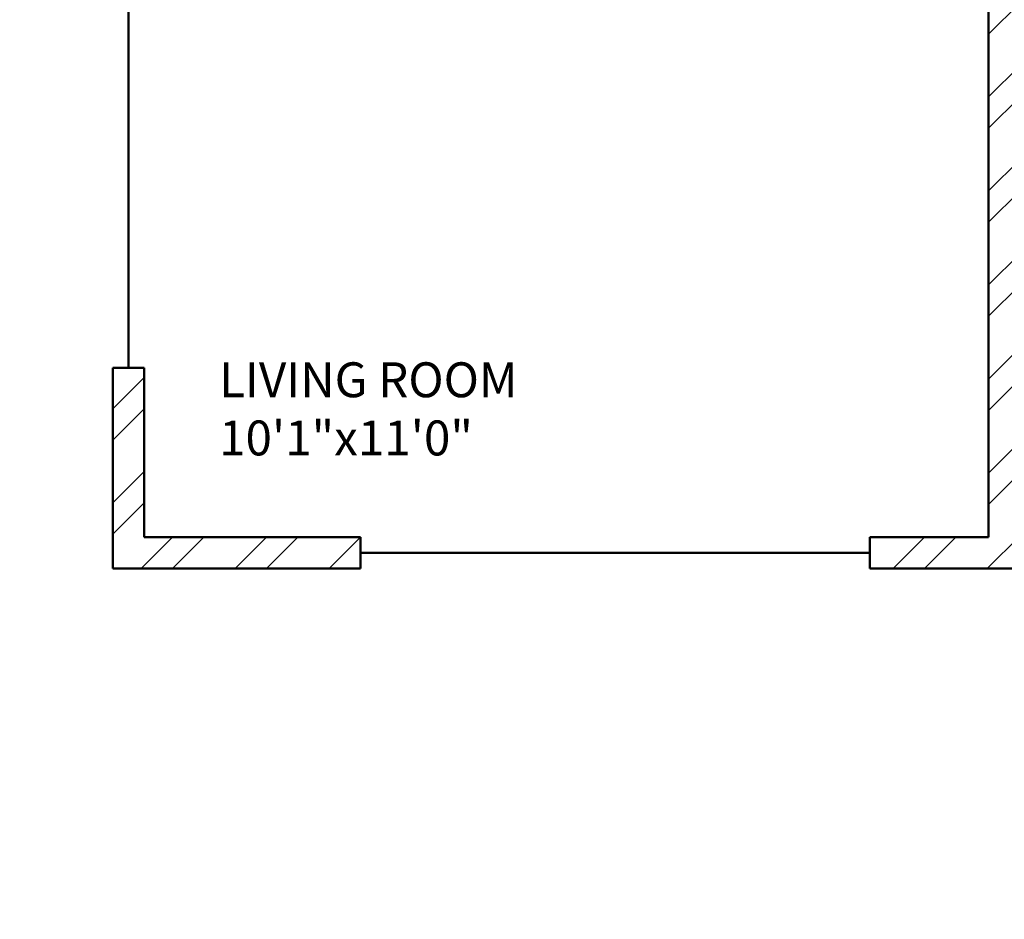
# Model space of a CAD drawing. Units: inches. Extents: x 1901 to 2863, y 888 to 2433.
# Tile 36 of 91: x 2477 to 2618, y 1474 to 1603. Entities that reach past the tile are written whole.
import ezdxf

# ---------------------------------------------------------------- set-up
doc = ezdxf.new("R2010")
doc.units = ezdxf.units.IN
for name, color, linetype, lineweight in [('A-AREA-IDEN', 7, 'Continuous', 18), ('A-WALL', 7, 'Continuous', 50), ('A-WALL-PATT', 8, 'Continuous', 13)]:
    doc.layers.add(name, color=color, linetype=linetype, lineweight=lineweight)
doc.styles.get("Standard").update_dxf_attribs({"font": 'arial.ttf'})

msp = doc.modelspace()

# ---------------------------------------------------------------- hatches: boundary and pattern name
at = {"layer": 'A-WALL-PATT'}
h = msp.add_hatch(dxfattribs=at)
h.set_pattern_fill('ANSI32', color=256)
h.paths.add_polyline_path([(2192.5, 2274.13), (2141.26, 2274.13), (2141.26, 2269.63), (2192.5, 2269.63)])
h.paths.add_polyline_path([(2259.93, 2274.13), (2216.5, 2274.13), (2216.5, 2269.63), (2255.43, 2269.63), (2255.43, 2214.63), (2250.81, 2214.63), (2250.81, 2210.13), (2259.93, 2210.13), (2259.93, 2215.13), (2271.76, 2215.13), (2271.76, 2217.38), (2271.76, 2219.63), (2259.93, 2219.63)])
h.paths.add_polyline_path([(2171.43, 2269.63), (2166.93, 2269.63), (2166.93, 2219.63), (2121.24, 2219.63), (2121.24, 2215.13), (2166.93, 2215.13), (2166.93, 2083.13), (2161.81, 2083.13), (2161.81, 2078.63), (2171.43, 2078.63), (2177, 2078.63), (2177, 2080.88), (2177, 2083.13), (2171.43, 2083.13), (2171.43, 2210.13), (2230.91, 2210.13), (2230.91, 2212.38), (2230.91, 2214.63), (2171.43, 2214.63)])
h.paths.add_polyline_path([(2117.26, 2274.13), (2089.43, 2274.13), (2089.43, 2219.63), (2081.14, 2219.63), (2081.14, 2215.13), (2089.43, 2215.13), (2098, 2215.13), (2098, 2217.38), (2098, 2219.63), (2093.93, 2219.63), (2093.93, 2269.63), (2117.26, 2269.63), (2117.26, 2271.88)])
h.paths.add_polyline_path([(2343.43, 2219.63), (2329.29, 2219.63), (2329.29, 2215.13), (2338.93, 2215.13), (2338.93, 2184.74), (2343.43, 2184.74)])
h.paths.add_polyline_path([(2338.93, 2083.13), (2329.29, 2083.13), (2208.97, 2083.13), (2208.97, 2078.63), (2338.93, 2078.63)])
h.paths.add_polyline_path([(2343.43, 2136.74), (2338.93, 2136.74), (2338.93, 1872.63), (2343.43, 1872.63)])
h.paths.add_polyline_path([(2343.43, 1863.63), (2397.68, 1863.63), (2397.68, 1821.63), (2384.14, 1821.63), (2384.14, 1812.63), (2418.33, 1812.63), (2418.33, 1817.13), (2418.33, 1821.63), (2406.68, 1821.63), (2406.68, 1863.63), (2459.5, 1863.63), (2459.5, 1821.63), (2447.14, 1821.63), (2447.14, 1812.63), (2459.5, 1812.63), (2468.5, 1812.63), (2468.5, 1872.63), (2394.43, 1872.63), (2334.43, 1872.63), (2334.43, 1812.63), (2343.43, 1812.63), (2353.25, 1812.63), (2353.25, 1821.63), (2343.43, 1821.63)])
h.paths.add_polyline_path([(2510.01, 1872.63), (2468.5, 1872.63), (2468.5, 1868.13), (2510.01, 1868.13)])
h.paths.add_polyline_path([(2514.01, 1817.13), (2468.5, 1817.13), (2468.5, 1812.63), (2482.11, 1812.63), (2482.11, 1800.61), (2486.61, 1800.61), (2486.61, 1812.63), (2514.01, 1812.63)])
h.paths.add_polyline_path([(2299.25, 1814.88), (2299.25, 1817.13), (2295.93, 1817.13), (2295.93, 1854.17), (2293.68, 1854.17), (2291.43, 1854.17), (2291.43, 1817.13), (2266.11, 1817.13), (2266.11, 1812.63), (2299.25, 1812.63)])
h.paths.add_polyline_path([(2218.11, 1817.13), (2206.46, 1817.13), (2171.43, 1817.13), (2171.43, 1949.13), (2190.1, 1949.13), (2190.1, 1953.63), (2163.47, 1953.63), (2163.47, 1949.13), (2166.93, 1949.13), (2166.93, 1817.13), (2114.3, 1817.13), (2114.3, 1812.63), (2218.11, 1812.63)])
h.paths.add_polyline_path([(2029.43, 1970.92), (2024.93, 1970.92), (2024.93, 1912.72), (2029.43, 1912.72)])
h.paths.add_polyline_path([(2132.3, 1953.63), (2113.93, 1953.63), (2113.93, 1975.89), (2111.68, 1975.89), (2109.43, 1975.89), (2109.43, 1953.63), (2029.43, 1953.63), (2029.43, 1949.13), (2132.3, 1949.13)])
h.paths.add_polyline_path([(2029.43, 1853.61), (2029.31, 1853.61), (2029.31, 1853.61), (2029.43, 1853.61), (2029.43, 1864.72), (2024.93, 1864.72), (2024.93, 1812.63), (2066.3, 1812.63), (2066.3, 1814.88), (2066.3, 1817.13), (2029.43, 1817.13)])
h.paths.add_polyline_path([(2122.93, 2010.09), (2120.68, 2010.09), (2118.43, 2010.09), (2118.43, 2006.13), (2029.43, 2006.13), (2029.43, 2001.63), (2109.43, 2001.63), (2109.43, 1998.04), (2113.93, 1998.04), (2113.93, 2001.63), (2122.93, 2001.63)])
h.paths.add_polyline_path([(2029.43, 2031.38), (2024.93, 2031.38), (2024.93, 1994.92), (2027.18, 1994.92), (2029.43, 1994.92)])
h.paths.add_polyline_path([(2029.43, 2136.74), (2024.93, 2136.74), (2024.93, 2067.38), (2027.18, 2067.38), (2029.43, 2067.38)])
h.paths.add_polyline_path([(2125.62, 2083.13), (2029.43, 2083.13), (2029.43, 2078.63), (2118.43, 2078.63), (2118.43, 2030.71), (2122.93, 2030.71), (2122.93, 2078.63), (2125.62, 2078.63)])
h.paths.add_polyline_path([(2029.43, 2215.13), (2040.47, 2215.13), (2040.47, 2217.38), (2040.47, 2219.63), (2024.93, 2219.63), (2024.93, 2184.74), (2029.43, 2184.74), (2029.43, 2187.78)])
h.paths.add_polyline_path([(2686.43, 2274.13), (2659.28, 2274.13), (2659.28, 2269.63), (2681.93, 2269.63), (2681.93, 2219.63), (2676.82, 2219.63), (2676.82, 2215.13), (2681.93, 2215.13), (2697.01, 2215.13), (2697.01, 2217.38), (2697.01, 2219.63), (2686.43, 2219.63)])
h.paths.add_polyline_path([(2609.93, 2269.63), (2635.28, 2269.63), (2635.28, 2274.13), (2571.43, 2274.13), (2571.43, 2269.63), (2605.43, 2269.63), (2605.43, 2214.63), (2549.1, 2214.63), (2549.1, 2210.13), (2605.43, 2210.13), (2605.43, 2083.13), (2601.01, 2083.13), (2601.01, 2080.88), (2601.01, 2078.63), (2609.93, 2078.63), (2616.16, 2078.63), (2616.16, 2080.88), (2616.16, 2083.13), (2609.93, 2083.13), (2609.93, 2215.13), (2651.46, 2215.13), (2651.46, 2217.38), (2651.46, 2219.63), (2609.93, 2219.63)])
h.paths.add_polyline_path([(2521.43, 2269.63), (2547.43, 2269.63), (2547.43, 2271.88), (2547.43, 2274.13), (2516.93, 2274.13), (2516.93, 2219.63), (2506.41, 2219.63), (2506.41, 2215.13), (2516.93, 2215.13), (2516.93, 2210.13), (2525.4, 2210.13), (2525.4, 2212.38), (2525.4, 2214.63), (2521.43, 2214.63)])
h.paths.add_polyline_path([(2456.01, 2219.63), (2439.43, 2219.63), (2439.43, 2187.89), (2443.93, 2187.89), (2443.93, 2215.13), (2456.01, 2215.13)])
h.paths.add_polyline_path([(2752.93, 2219.63), (2739.48, 2219.63), (2739.48, 2215.13), (2748.43, 2215.13), (2748.43, 2187.89), (2752.93, 2187.89)])
h.paths.add_polyline_path([(2752.93, 2139.89), (2748.43, 2139.89), (2748.43, 2083.13), (2648.42, 2083.13), (2648.42, 2078.63), (2654.93, 2078.63), (2654.93, 2039.44), (2659.43, 2039.44), (2659.43, 2078.63), (2748.43, 2078.63), (2748.43, 2063.43), (2752.93, 2063.43)])
h.paths.add_polyline_path([(2752.93, 2010.63), (2659.43, 2010.63), (2659.43, 2015.65), (2654.93, 2015.65), (2654.93, 2010.63), (2605.43, 2010.63), (2605.43, 1920.97), (2609.93, 1920.97), (2609.93, 2006.13), (2748.43, 2006.13), (2748.43, 1982.47), (2752.93, 1982.47)])
h.paths.add_polyline_path([(2752.93, 2027.43), (2748.43, 2027.43), (2748.43, 2010.63), (2752.93, 2010.63)])
h.paths.add_polyline_path([(2748.43, 1886.13), (2609.93, 1886.13), (2609.93, 1889.72), (2605.43, 1889.72), (2605.43, 1861.26), (2609.93, 1861.26), (2609.93, 1881.63), (2748.43, 1881.63)])
h.paths.add_polyline_path([(2456.86, 2228.83), (2498.4, 2228.83), (2498.4, 2247.49), (2456.86, 2247.49)], flags=9)
h.paths.add_polyline_path([(2038.6, 2237.42), (2080.17, 2237.42), (2080.17, 2256.08), (2038.6, 2256.08)], flags=9)
h.paths.add_polyline_path([(2292.01, 1062.39), (2539.93, 1062.39), (2539.93, 1099.49), (2292.01, 1099.49)], flags=9)
h.paths.add_polyline_path([(2424.91, 1832.25), (2448.51, 1832.25), (2448.51, 1846.68), (2424.91, 1846.68)], flags=25)
h.paths.add_polyline_path([(2359.08, 1832.25), (2382.68, 1832.25), (2382.68, 1846.68), (2359.08, 1846.68)], flags=25)
h.paths.add_polyline_path([(2352.9, 1684.8), (2367.54, 1684.8), (2367.54, 1697.17), (2352.9, 1697.17)], flags=9)
h.paths.add_polyline_path([(2079.29, 1755.83), (2169.02, 1755.83), (2169.02, 1774.37), (2079.29, 1774.37)], flags=9)
h.paths.add_polyline_path([(2404.09, 1373.86), (2404.09, 1463.59), (2385.54, 1463.59), (2385.54, 1373.86)], flags=9)
h.paths.add_polyline_path([(2268.09, 2236.37), (2309.64, 2236.37), (2309.64, 2255.03), (2268.09, 2255.03)], flags=9)
h.paths.add_polyline_path([(2575.96, 1700.95), (2665.7, 1700.95), (2665.7, 1719.5), (2575.96, 1719.5)], flags=9)
h.paths.add_polyline_path([(2302.96, 1878.47), (2329.52, 1878.47), (2329.52, 1888.78), (2302.96, 1888.78)], flags=9)
h.paths.add_polyline_path([(2097.42, 2240.58), (2126.57, 2240.58), (2126.57, 2259.23), (2097.42, 2259.23)], flags=9)
h.paths.add_polyline_path([(2208.72, 2246.12), (2237.88, 2246.12), (2237.88, 2264.78), (2208.72, 2264.78)], flags=9)
h.paths.add_polyline_path([(2038.15, 1925.96), (2076.99, 1925.96), (2076.99, 1944.62), (2038.15, 1944.62)], flags=9)
h.paths.add_polyline_path([(2239.14, 1926.67), (2288.46, 1926.67), (2288.46, 1945.33), (2239.14, 1945.33)], flags=9)
h.paths.add_polyline_path([(2175.43, 2007.33), (2212.36, 2007.33), (2212.36, 2025.99), (2175.43, 2025.99)], flags=9)
h.paths.add_polyline_path([(2225.03, 2091.79), (2263.87, 2091.79), (2263.87, 2110.45), (2225.03, 2110.45)], flags=9)
h.paths.add_polyline_path([(2035.4, 2098.48), (2074.24, 2098.48), (2074.24, 2117.14), (2035.4, 2117.14)], flags=9)
h.paths.add_polyline_path([(2050.1, 2029.21), (2083.26, 2029.21), (2083.26, 2047.87), (2050.1, 2047.87)], flags=9)
h.paths.add_polyline_path([(2069.68, 1956.72), (2098.83, 1956.72), (2098.83, 1975.38), (2069.68, 1975.38)], flags=25)
h.paths.add_polyline_path([(2328.62, 1753.34), (2361.66, 1753.34), (2361.66, 1771.99), (2328.62, 1771.99)], flags=9)
h.paths.add_polyline_path([(2395.16, 2060.89), (2395.16, 2140.65), (2378.68, 2140.65), (2378.68, 2060.89)], flags=9)
h.paths.add_polyline_path([(2463.73, 2059.02), (2492.89, 2059.02), (2492.89, 2077.68), (2463.73, 2077.68)], flags=9)
h.paths.add_polyline_path([(2458.03, 2181.54), (2496.87, 2181.54), (2496.87, 2200.19), (2458.03, 2200.19)], flags=9)
h.paths.add_polyline_path([(2527.58, 2243.07), (2556.73, 2243.07), (2556.73, 2261.73), (2527.58, 2261.73)], flags=9)
h.paths.add_polyline_path([(2694.46, 2232.77), (2736.03, 2232.77), (2736.03, 2251.42), (2694.46, 2251.42)], flags=9)
h.paths.add_polyline_path([(2637.82, 2249.22), (2666.98, 2249.22), (2666.98, 2267.88), (2637.82, 2267.88)], flags=9)
h.paths.add_polyline_path([(2623.69, 2183.54), (2662.53, 2183.54), (2662.53, 2202.2), (2623.69, 2202.2)], flags=9)
h.paths.add_polyline_path([(2691.97, 2021.5), (2725.12, 2021.5), (2725.12, 2040.16), (2691.97, 2040.16)], flags=9)
h.paths.add_polyline_path([(2621.04, 1975.91), (2662.34, 1975.91), (2662.34, 1994.57), (2621.04, 1994.57)], flags=25)
h.paths.add_polyline_path([(2479.03, 1927.62), (2519.84, 1927.62), (2519.84, 1946.28), (2479.03, 1946.28)], flags=9)
h.paths.add_polyline_path([(2670.94, 1849.08), (2716.01, 1849.08), (2716.01, 1867.73), (2670.94, 1867.73)], flags=9)
h.paths.add_polyline_path([(2523.61, 1782.96), (2550.17, 1782.96), (2550.17, 1793.26), (2523.61, 1793.26)], flags=9)
h.paths.add_polyline_path([(2450.84, 1207.33), (2492.39, 1207.33), (2492.39, 1225.99), (2450.84, 1225.99)], flags=9)
h.paths.add_polyline_path([(2527.75, 1203.84), (2556.91, 1203.84), (2556.91, 1222.5), (2527.75, 1222.5)], flags=9)
h.paths.add_polyline_path([(2639.11, 1207.2), (2668.27, 1207.2), (2668.27, 1225.86), (2639.11, 1225.86)], flags=9)
h.paths.add_polyline_path([(2692.59, 1218.97), (2734.17, 1218.97), (2734.17, 1237.62), (2692.59, 1237.62)], flags=9)
h.paths.add_polyline_path([(2669.27, 1366.33), (2708.11, 1366.33), (2708.11, 1384.99), (2669.27, 1384.99)], flags=9)
h.paths.add_polyline_path([(2463.31, 1358.03), (2502.15, 1358.03), (2502.15, 1376.69), (2463.31, 1376.69)], flags=9)
h.paths.add_polyline_path([(2494.72, 1449.96), (2531.65, 1449.96), (2531.65, 1468.62), (2494.72, 1468.62)], flags=9)
h.paths.add_polyline_path([(2675.57, 1422.16), (2708.72, 1422.16), (2708.72, 1440.81), (2675.57, 1440.81)], flags=9)
h.paths.add_polyline_path([(2685.63, 1493.89), (2714.79, 1493.89), (2714.79, 1512.55), (2685.63, 1512.55)], flags=9)
h.paths.add_polyline_path([(2686.8, 1529.91), (2725.65, 1529.91), (2725.65, 1548.57), (2686.8, 1548.57)], flags=9)
h.paths.add_polyline_path([(2503.65, 1537.99), (2552.97, 1537.99), (2552.97, 1556.65), (2503.65, 1556.65)], flags=9)
h.paths.add_polyline_path([(2291.71, 1643.5), (2318.28, 1643.5), (2318.28, 1653.81), (2291.71, 1653.81)], flags=9)
h.paths.add_polyline_path([(2450.63, 1610.52), (2477.19, 1610.52), (2477.19, 1620.82), (2450.63, 1620.82)], flags=9)
h.paths.add_polyline_path([(2359.99, 1551.81), (2422.25, 1551.81), (2422.25, 1562.12), (2359.99, 1562.12)], flags=9)
h.paths.add_polyline_path([(2280.11, 1249.01), (2321.65, 1249.01), (2321.65, 1267.66), (2280.11, 1267.66)], flags=9)
h.paths.add_polyline_path([(2164.06, 1274.23), (2193.22, 1274.23), (2193.22, 1292.89), (2164.06, 1292.89)], flags=9)
h.paths.add_polyline_path([(2118.21, 1277.69), (2151.25, 1277.69), (2151.25, 1296.35), (2118.21, 1296.35)], flags=9)
h.paths.add_polyline_path([(2031.95, 1268.53), (2073.52, 1268.53), (2073.52, 1287.19), (2031.95, 1287.19)], flags=9)
h.paths.add_polyline_path([(2050.2, 1409.08), (2089.04, 1409.08), (2089.04, 1427.74), (2050.2, 1427.74)], flags=9)
h.paths.add_polyline_path([(2243.74, 1421.03), (2282.58, 1421.03), (2282.58, 1439.69), (2243.74, 1439.69)], flags=9)
h.paths.add_polyline_path([(2190.75, 1509.77), (2231.56, 1509.77), (2231.56, 1528.43), (2190.75, 1528.43)], flags=9)
h.paths.add_polyline_path([(2058.39, 1475.42), (2091.55, 1475.42), (2091.55, 1494.07), (2058.39, 1494.07)], flags=9)
h.paths.add_polyline_path([(2062.45, 1553.09), (2091.6, 1553.09), (2091.6, 1571.75), (2062.45, 1571.75)], flags=9)
h.paths.add_polyline_path([(2219.52, 1590.37), (2266.15, 1590.37), (2266.15, 1609.02), (2219.52, 1609.02)], flags=9)
h.paths.add_polyline_path([(2041.07, 1584.19), (2079.91, 1584.19), (2079.91, 1602.85), (2041.07, 1602.85)], flags=9)
h = msp.add_hatch(dxfattribs=at)
h.set_pattern_fill('ANSI32', color=256)
h.paths.add_polyline_path([(2443.93, 2139.89), (2439.43, 2139.89), (2439.43, 2069.35), (2441.68, 2069.35), (2443.93, 2069.35), (2443.93, 2078.63), (2521.93, 2078.63), (2521.93, 2075.07), (2524.18, 2075.07), (2526.43, 2075.07), (2526.43, 2078.63), (2571.75, 2078.63), (2571.75, 2080.88), (2571.75, 2083.13), (2443.93, 2083.13)])
h.paths.add_polyline_path([(2526.43, 2054.63), (2524.18, 2054.63), (2521.93, 2054.63), (2521.93, 2030.63), (2443.93, 2030.63), (2443.93, 2045.35), (2439.43, 2045.35), (2439.43, 1983.87), (2443.93, 1983.87), (2443.93, 2026.13), (2521.93, 2026.13), (2526.43, 2026.13)])
h.paths.add_polyline_path([(2443.93, 1923.87), (2439.43, 1923.87), (2439.43, 1872.63), (2443.93, 1872.63)])
h.paths.add_polyline_path([(2636.23, 1766.13), (2609.93, 1766.13), (2609.93, 1779.79), (2605.43, 1779.79), (2605.43, 1766.13), (2486.61, 1766.13), (2486.61, 1770.67), (2482.11, 1770.67), (2482.11, 1766.13), (2482.11, 1761.63), (2636.23, 1761.63), (2636.23, 1763.88)])
h.paths.add_polyline_path([(2519.54, 1663.38), (2519.54, 1665.63), (2494.93, 1665.63), (2481.83, 1665.63), (2481.83, 1663.38), (2481.83, 1661.13), (2490.43, 1661.13), (2490.43, 1640.16), (2494.93, 1640.16), (2494.93, 1661.13), (2519.54, 1661.13)])
h.paths.add_polyline_path([(2443.93, 1712.13), (2443.93, 1716.63), (2414.46, 1716.63), (2414.46, 1712.13), (2439.43, 1712.13), (2439.43, 1545.51), (2443.93, 1545.51), (2443.93, 1661.13), (2448.47, 1661.13), (2448.47, 1665.63), (2443.93, 1665.63)])
h.paths.add_polyline_path([(2343.43, 1712.13), (2365.52, 1712.13), (2365.52, 1714.38), (2365.52, 1716.63), (2333.87, 1716.63), (2333.87, 1714.38), (2333.87, 1712.13), (2338.93, 1712.13), (2338.93, 1575.63), (2338.93, 1545.51), (2343.43, 1545.51), (2343.43, 1547.51), (2343.43, 1580.13)])
h.paths.add_polyline_path([(2752.93, 1665.63), (2579.54, 1665.63), (2579.54, 1661.13), (2615.93, 1661.13), (2615.93, 1529.13), (2598.93, 1529.13), (2598.93, 1524.63), (2623.13, 1524.63), (2623.13, 1526.88), (2623.13, 1529.13), (2620.43, 1529.13), (2620.43, 1661.13), (2748.43, 1661.13), (2748.43, 1633.5), (2752.93, 1633.5)])
h.paths.add_polyline_path([(2752.93, 1419.93), (2748.43, 1419.93), (2748.43, 1400.13), (2659.43, 1400.13), (2659.43, 1444.33), (2657.18, 1444.33), (2654.93, 1444.33), (2654.93, 1400.13), (2643.65, 1400.13), (2643.65, 1395.63), (2748.43, 1395.63), (2748.43, 1364.04), (2752.93, 1364.04)])
h.paths.add_polyline_path([(2752.93, 1492.88), (2748.43, 1492.88), (2748.43, 1476.63), (2667.43, 1476.63), (2667.43, 1479.71), (2665.18, 1479.71), (2662.93, 1479.71), (2662.93, 1476.63), (2654.93, 1476.63), (2654.93, 1469.54), (2659.43, 1469.54), (2659.43, 1472.13), (2748.43, 1472.13), (2748.43, 1455.93), (2752.93, 1455.93)])
h.paths.add_polyline_path([(2752.93, 1304.04), (2748.43, 1304.04), (2748.43, 1263.63), (2738.66, 1263.63), (2738.66, 1259.13), (2752.93, 1259.13)])
h.paths.add_polyline_path([(2685.93, 1259.13), (2695.49, 1259.13), (2695.49, 1261.38), (2695.49, 1263.63), (2677.84, 1263.63), (2677.84, 1261.38), (2677.84, 1259.13), (2681.43, 1259.13), (2681.43, 1203.63), (2653.28, 1203.63), (2653.28, 1199.13), (2685.93, 1199.13), (2685.93, 1203.63)])
h.paths.add_polyline_path([(2609.43, 1395.63), (2611.85, 1395.63), (2611.85, 1400.13), (2598.89, 1400.13), (2598.89, 1397.88), (2598.89, 1395.63), (2604.93, 1395.63), (2604.93, 1268.13), (2554.73, 1268.13), (2554.73, 1265.88), (2554.73, 1263.63), (2604.93, 1263.63), (2604.93, 1203.63), (2571.31, 1203.63), (2571.31, 1199.13), (2604.93, 1199.13), (2629.28, 1199.13), (2629.28, 1201.38), (2629.28, 1203.63), (2609.43, 1203.63), (2609.43, 1258.63), (2609.43, 1259.13), (2654.8, 1259.13), (2654.8, 1263.63), (2609.43, 1263.63)])
h.paths.add_polyline_path([(2443.93, 1304.04), (2439.43, 1304.04), (2439.43, 1259.13), (2443.93, 1259.13), (2456.16, 1259.13), (2456.16, 1261.38), (2456.16, 1263.63), (2443.93, 1263.63)])
h.paths.add_polyline_path([(2525.43, 1263.63), (2531.78, 1263.63), (2531.78, 1268.13), (2520.93, 1268.13), (2520.93, 1263.63), (2511.41, 1263.63), (2511.41, 1259.13), (2520.93, 1259.13), (2520.93, 1199.13), (2547.31, 1199.13), (2547.31, 1201.38), (2547.31, 1203.63), (2525.43, 1203.63)])
h.paths.add_polyline_path([(2443.93, 1434.84), (2439.43, 1434.84), (2439.43, 1364.04), (2441.68, 1364.04), (2443.93, 1364.04)])
h.paths.add_polyline_path([(2567.13, 1400.13), (2443.93, 1400.13), (2443.93, 1395.63), (2567.13, 1395.63)])
h.paths.add_polyline_path([(2443.93, 1545.51), (2439.43, 1545.51), (2439.43, 1494.84), (2443.93, 1494.84)])
h.paths.add_polyline_path([(2494.93, 1553.35), (2492.68, 1553.35), (2490.43, 1553.35), (2490.43, 1524.63), (2494.93, 1524.63), (2525.94, 1524.63), (2525.94, 1526.88), (2525.94, 1529.13), (2494.93, 1529.13)])
h.paths.add_polyline_path([(2752.93, 1573.5), (2748.43, 1573.5), (2748.43, 1529.13), (2657.76, 1529.13), (2657.76, 1524.63), (2662.93, 1524.63), (2662.93, 1498.63), (2667.43, 1498.63), (2667.43, 1524.63), (2748.43, 1524.63), (2748.43, 1516.88), (2752.93, 1516.88)])
h.paths.add_polyline_path([(2038.6, 2237.42), (2080.17, 2237.42), (2080.17, 2256.08), (2038.6, 2256.08)], flags=9)
h.paths.add_polyline_path([(2292.01, 1062.39), (2539.93, 1062.39), (2539.93, 1099.49), (2292.01, 1099.49)], flags=9)
h.paths.add_polyline_path([(2424.91, 1832.25), (2448.51, 1832.25), (2448.51, 1846.68), (2424.91, 1846.68)], flags=9)
h.paths.add_polyline_path([(2359.08, 1832.25), (2382.68, 1832.25), (2382.68, 1846.68), (2359.08, 1846.68)], flags=9)
h.paths.add_polyline_path([(2352.9, 1684.8), (2367.54, 1684.8), (2367.54, 1697.17), (2352.9, 1697.17)], flags=9)
h.paths.add_polyline_path([(2079.29, 1755.83), (2169.02, 1755.83), (2169.02, 1774.37), (2079.29, 1774.37)], flags=9)
h.paths.add_polyline_path([(2404.09, 1373.86), (2404.09, 1463.59), (2385.54, 1463.59), (2385.54, 1373.86)], flags=9)
h.paths.add_polyline_path([(2268.09, 2236.37), (2309.64, 2236.37), (2309.64, 2255.03), (2268.09, 2255.03)], flags=9)
h.paths.add_polyline_path([(2575.96, 1700.95), (2665.7, 1700.95), (2665.7, 1719.5), (2575.96, 1719.5)], flags=9)
h.paths.add_polyline_path([(2302.96, 1878.47), (2329.52, 1878.47), (2329.52, 1888.78), (2302.96, 1888.78)], flags=9)
h.paths.add_polyline_path([(2097.42, 2240.58), (2126.57, 2240.58), (2126.57, 2259.23), (2097.42, 2259.23)], flags=9)
h.paths.add_polyline_path([(2208.72, 2246.12), (2237.88, 2246.12), (2237.88, 2264.78), (2208.72, 2264.78)], flags=9)
h.paths.add_polyline_path([(2038.15, 1925.96), (2076.99, 1925.96), (2076.99, 1944.62), (2038.15, 1944.62)], flags=9)
h.paths.add_polyline_path([(2239.14, 1926.67), (2288.46, 1926.67), (2288.46, 1945.33), (2239.14, 1945.33)], flags=9)
h.paths.add_polyline_path([(2175.43, 2007.33), (2212.36, 2007.33), (2212.36, 2025.99), (2175.43, 2025.99)], flags=9)
h.paths.add_polyline_path([(2225.03, 2091.79), (2263.87, 2091.79), (2263.87, 2110.45), (2225.03, 2110.45)], flags=9)
h.paths.add_polyline_path([(2035.4, 2098.48), (2074.24, 2098.48), (2074.24, 2117.14), (2035.4, 2117.14)], flags=9)
h.paths.add_polyline_path([(2050.1, 2029.21), (2083.26, 2029.21), (2083.26, 2047.87), (2050.1, 2047.87)], flags=9)
h.paths.add_polyline_path([(2069.68, 1956.72), (2098.83, 1956.72), (2098.83, 1975.38), (2069.68, 1975.38)], flags=9)
h.paths.add_polyline_path([(2328.62, 1753.34), (2361.66, 1753.34), (2361.66, 1771.99), (2328.62, 1771.99)], flags=9)
h.paths.add_polyline_path([(2395.16, 2060.89), (2395.16, 2140.65), (2378.68, 2140.65), (2378.68, 2060.89)], flags=9)
h.paths.add_polyline_path([(2463.73, 2059.02), (2492.89, 2059.02), (2492.89, 2077.68), (2463.73, 2077.68)], flags=9)
h.paths.add_polyline_path([(2458.03, 2181.54), (2496.87, 2181.54), (2496.87, 2200.19), (2458.03, 2200.19)], flags=9)
h.paths.add_polyline_path([(2456.86, 2228.83), (2498.4, 2228.83), (2498.4, 2247.49), (2456.86, 2247.49)], flags=9)
h.paths.add_polyline_path([(2527.58, 2243.07), (2556.73, 2243.07), (2556.73, 2261.73), (2527.58, 2261.73)], flags=9)
h.paths.add_polyline_path([(2694.46, 2232.77), (2736.03, 2232.77), (2736.03, 2251.42), (2694.46, 2251.42)], flags=9)
h.paths.add_polyline_path([(2637.82, 2249.22), (2666.98, 2249.22), (2666.98, 2267.88), (2637.82, 2267.88)], flags=9)
h.paths.add_polyline_path([(2623.69, 2183.54), (2662.53, 2183.54), (2662.53, 2202.2), (2623.69, 2202.2)], flags=9)
h.paths.add_polyline_path([(2691.97, 2021.5), (2725.12, 2021.5), (2725.12, 2040.16), (2691.97, 2040.16)], flags=9)
h.paths.add_polyline_path([(2621.04, 1975.91), (2662.34, 1975.91), (2662.34, 1994.57), (2621.04, 1994.57)], flags=9)
h.paths.add_polyline_path([(2479.03, 1927.62), (2519.84, 1927.62), (2519.84, 1946.28), (2479.03, 1946.28)], flags=9)
h.paths.add_polyline_path([(2670.94, 1849.08), (2716.01, 1849.08), (2716.01, 1867.73), (2670.94, 1867.73)], flags=9)
h.paths.add_polyline_path([(2523.61, 1782.96), (2550.17, 1782.96), (2550.17, 1793.26), (2523.61, 1793.26)], flags=9)
h.paths.add_polyline_path([(2450.84, 1207.33), (2492.39, 1207.33), (2492.39, 1225.99), (2450.84, 1225.99)], flags=9)
h.paths.add_polyline_path([(2527.75, 1203.84), (2556.91, 1203.84), (2556.91, 1222.5), (2527.75, 1222.5)], flags=9)
h.paths.add_polyline_path([(2639.11, 1207.2), (2668.27, 1207.2), (2668.27, 1225.86), (2639.11, 1225.86)], flags=9)
h.paths.add_polyline_path([(2692.59, 1218.97), (2734.17, 1218.97), (2734.17, 1237.62), (2692.59, 1237.62)], flags=9)
h.paths.add_polyline_path([(2669.27, 1366.33), (2708.11, 1366.33), (2708.11, 1384.99), (2669.27, 1384.99)], flags=25)
h.paths.add_polyline_path([(2463.31, 1358.03), (2502.15, 1358.03), (2502.15, 1376.69), (2463.31, 1376.69)], flags=9)
h.paths.add_polyline_path([(2494.72, 1449.96), (2531.65, 1449.96), (2531.65, 1468.62), (2494.72, 1468.62)], flags=9)
h.paths.add_polyline_path([(2675.57, 1422.16), (2708.72, 1422.16), (2708.72, 1440.81), (2675.57, 1440.81)], flags=25)
h.paths.add_polyline_path([(2685.63, 1493.89), (2714.79, 1493.89), (2714.79, 1512.55), (2685.63, 1512.55)], flags=9)
h.paths.add_polyline_path([(2686.8, 1529.91), (2725.65, 1529.91), (2725.65, 1548.57), (2686.8, 1548.57)], flags=25)
h.paths.add_polyline_path([(2503.65, 1537.99), (2552.97, 1537.99), (2552.97, 1556.65), (2503.65, 1556.65)], flags=9)
h.paths.add_polyline_path([(2291.71, 1643.5), (2318.28, 1643.5), (2318.28, 1653.81), (2291.71, 1653.81)], flags=9)
h.paths.add_polyline_path([(2450.63, 1610.52), (2477.19, 1610.52), (2477.19, 1620.82), (2450.63, 1620.82)], flags=9)
h.paths.add_polyline_path([(2359.99, 1551.81), (2422.25, 1551.81), (2422.25, 1562.12), (2359.99, 1562.12)], flags=9)
h.paths.add_polyline_path([(2280.11, 1249.01), (2321.65, 1249.01), (2321.65, 1267.66), (2280.11, 1267.66)], flags=9)
h.paths.add_polyline_path([(2164.06, 1274.23), (2193.22, 1274.23), (2193.22, 1292.89), (2164.06, 1292.89)], flags=9)
h.paths.add_polyline_path([(2118.21, 1277.69), (2151.25, 1277.69), (2151.25, 1296.35), (2118.21, 1296.35)], flags=9)
h.paths.add_polyline_path([(2031.95, 1268.53), (2073.52, 1268.53), (2073.52, 1287.19), (2031.95, 1287.19)], flags=9)
h.paths.add_polyline_path([(2050.2, 1409.08), (2089.04, 1409.08), (2089.04, 1427.74), (2050.2, 1427.74)], flags=9)
h.paths.add_polyline_path([(2243.74, 1421.03), (2282.58, 1421.03), (2282.58, 1439.69), (2243.74, 1439.69)], flags=9)
h.paths.add_polyline_path([(2190.75, 1509.77), (2231.56, 1509.77), (2231.56, 1528.43), (2190.75, 1528.43)], flags=9)
h.paths.add_polyline_path([(2058.39, 1475.42), (2091.55, 1475.42), (2091.55, 1494.07), (2058.39, 1494.07)], flags=9)
h.paths.add_polyline_path([(2062.45, 1553.09), (2091.6, 1553.09), (2091.6, 1571.75), (2062.45, 1571.75)], flags=9)
h.paths.add_polyline_path([(2219.52, 1590.37), (2266.15, 1590.37), (2266.15, 1609.02), (2219.52, 1609.02)], flags=9)
h.paths.add_polyline_path([(2041.07, 1584.19), (2079.91, 1584.19), (2079.91, 1602.85), (2041.07, 1602.85)], flags=9)

# ---------------------------------------------------------------- linework, layer by layer
at = {"layer": 'A-WALL'}
for p, q in [((2615.93, 1529.13), (2615.93, 1661.13)), ((2492.68, 1553.35), (2492.68, 1640.16)), ((2490.43, 1524.63), (2490.43, 1553.35)), ((2490.43, 1553.35), (2494.93, 1553.35)), ((2494.93, 1553.35), (2492.68, 1553.35)), ((2494.93, 1553.35), (2494.93, 1529.13)), ((2494.93, 1529.13), (2525.94, 1529.13)), ((2525.94, 1529.13), (2525.94, 1524.63)), ((2598.93, 1526.88), (2598.93, 1529.13)), ((2598.93, 1529.13), (2598.93, 1524.63)), ((2598.93, 1529.13), (2615.93, 1529.13)), ((2525.94, 1524.63), (2525.94, 1526.88)), ((2525.94, 1526.88), (2598.93, 1526.88)), ((2490.43, 1524.63), (2525.94, 1524.63)), ((2494.93, 1524.63), (2490.43, 1524.63)), ((2598.93, 1524.63), (2623.13, 1524.63)), ((2620.43, 1524.63), (2615.93, 1524.63))]:
    msp.add_line(p, q, dxfattribs=at)

# ---------------------------------------------------------------- texts
at = {"layer": 'A-AREA-IDEN', "insert": (2505.66, 1554.16), "char_height": 5, "attachment_point": 1}
msp.add_mtext_dynamic_manual_height_columns('LIVING ROOM\\P10\'1"x11\'0"', width=202.8676, gutter_width=12.5, heights=[0], dxfattribs=at)

doc.saveas('drawing.dxf')
